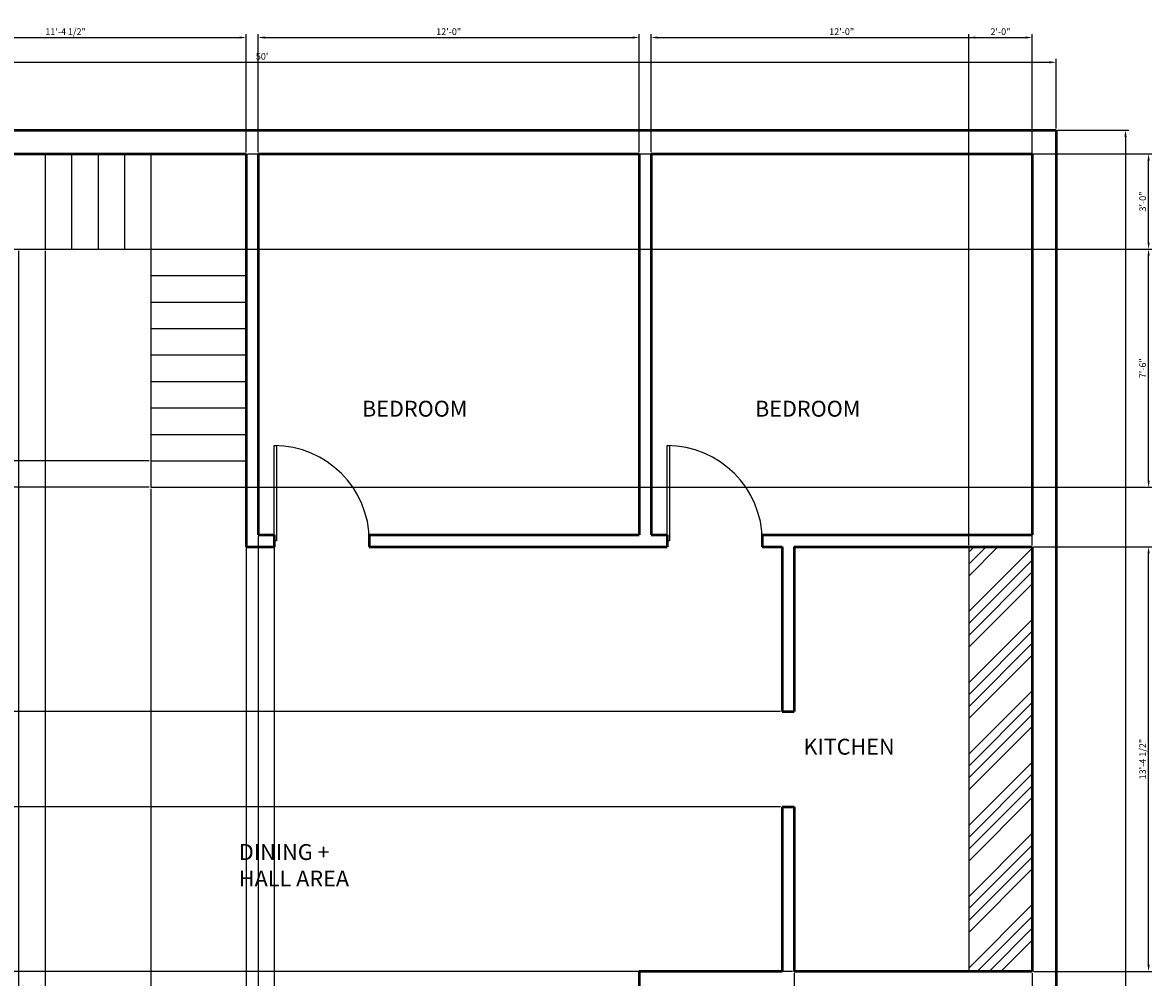
# Model space of a CAD drawing. Units: inches. Extents: x 877 to 2164, y 771 to 1603.
# Tile 4 of 6: x 1281 to 1709, y 1177 to 1538. Entities that reach past the tile are written whole.
import ezdxf

# ---------------------------------------------------------------- set-up
doc = ezdxf.new("R2010")
doc.units = ezdxf.units.IN
for name, color, linetype, lineweight in [('A-ANNO-DIMS', 2, 'Continuous', 18), ('A-AREA-IDEN', 7, 'Continuous', 25), ('A-DOOR', 5, 'Continuous', 25), ('A-FLOR-CASE', 8, 'Continuous', 25), ('A-FLOR-CASE-PATT', 252, 'Continuous', 13), ('A-FLOR-STRS', 7, 'Continuous', 25), ('A-WALL', 7, 'Continuous', 50)]:
    doc.layers.add(name, color=color, linetype=linetype, lineweight=lineweight)
doc.styles.get("Standard").update_dxf_attribs({"font": 'arial.ttf'})
doc.dimstyles.new('ISO-25', dxfattribs={"dimtxt": 2.5, "dimasz": 2.5, "dimexe": 1.25, "dimexo": 0.625, "dimtad": 1, "dimdec": 0, "dimlunit": 4, "dimtxsty": 'Standard', "dimcen": 2.5, "dimadec": 0, "dimazin": 0, "dimtfac": 1, "dimtdec": 0, "dimtmove": 0, "dimatfit": 3, "dimfxl": 1, "dimarcsym": 0})

# ---------------------------------------------------------------- blocks, each defined once
blk = doc.blocks.new('*D1')
at = {"layer": 'A-ANNO-DIMS', "color": 0, "lineweight": -2, "transparency": 16777216}
for p, q in [((1071.89, 1498.25), (1071.89, 1524.5)), ((1074.39, 1523.25), (1669.39, 1523.25)), ((1671.89, 1498.25), (1671.89, 1524.5))]:
    blk.add_line(p, q, dxfattribs=at)
at = {"layer": 'A-ANNO-DIMS', "color": 0, "transparency": 16777216}
for points in [[(1074.39, 1523.66), (1074.39, 1522.83), (1071.89, 1523.25)], [(1669.39, 1523.66), (1669.39, 1522.83), (1671.89, 1523.25)]]:
    blk.add_solid(points, dxfattribs=at)
at = {"layer": 'Defpoints', "color": 0, "transparency": 16777216}
for p in [(1671.89, 1523.25), (1071.89, 1497.62), (1671.89, 1497.62)]:
    blk.add_point(p, dxfattribs=at)
at = {"layer": 'A-ANNO-DIMS', "color": 0, "transparency": 16777216, "insert": (1371.89, 1525.15), "char_height": 2.5, "attachment_point": 5}
blk.add_mtext("50'", dxfattribs=at)
blk = doc.blocks.new('*D2')
at = {"layer": 'A-ANNO-DIMS', "color": 0, "lineweight": -2, "transparency": 16777216}
for p, q in [((1672.52, 1497.62), (1699.4, 1497.62)), ((1698.15, 1495.12), (1698.15, 840.12)), ((1672.52, 837.62), (1699.4, 837.62))]:
    blk.add_line(p, q, dxfattribs=at)
at = {"layer": 'A-ANNO-DIMS', "color": 0, "transparency": 16777216}
for points in [[(1697.73, 1495.12), (1698.57, 1495.12), (1698.15, 1497.62)], [(1697.73, 840.12), (1698.57, 840.12), (1698.15, 837.62)]]:
    blk.add_solid(points, dxfattribs=at)
at = {"layer": 'Defpoints', "color": 0, "transparency": 16777216}
for p in [(1671.89, 1497.62), (1671.89, 837.62), (1698.15, 837.62)]:
    blk.add_point(p, dxfattribs=at)
at = {"layer": 'A-ANNO-DIMS', "color": 0, "transparency": 16777216, "insert": (1696.26, 1167.62), "char_height": 2.5, "attachment_point": 5, "rotation": 90}
blk.add_mtext("55'", dxfattribs=at)
blk = doc.blocks.new('DOOR-SINGLE-36IN')
blk.add_lwpolyline([(0, 0), (0, 1), (36, 1), (36, 0)], close=True)
blk.add_arc((36, 0), 36, 90, 180)
blk = doc.blocks.new('*D11')
at = {"layer": 'A-ANNO-DIMS', "color": 0, "lineweight": -2, "transparency": 16777216}
for p, q in [((1229.39, 1489.25), (1229.39, 1533.85)), ((1231.89, 1532.6), (1363.39, 1532.6)), ((1365.89, 1489.25), (1365.89, 1533.85))]:
    blk.add_line(p, q, dxfattribs=at)
at = {"layer": 'A-ANNO-DIMS', "color": 0, "transparency": 16777216}
for points in [[(1231.89, 1533.01), (1231.89, 1532.18), (1229.39, 1532.6)], [(1363.39, 1533.01), (1363.39, 1532.18), (1365.89, 1532.6)]]:
    blk.add_solid(points, dxfattribs=at)
at = {"layer": 'Defpoints', "color": 0, "transparency": 16777216}
for p in [(1365.89, 1532.6), (1229.39, 1488.62), (1365.89, 1488.62)]:
    blk.add_point(p, dxfattribs=at)
at = {"layer": 'A-ANNO-DIMS', "color": 0, "transparency": 16777216, "insert": (1297.64, 1534.51), "char_height": 2.5, "attachment_point": 5}
blk.add_mtext('11\'-4 1/2"', dxfattribs=at)
blk = doc.blocks.new('*D12')
at = {"layer": 'A-ANNO-DIMS', "color": 0, "lineweight": -2, "transparency": 16777216}
for p, q in [((1370.39, 1489.25), (1370.39, 1533.85)), ((1372.89, 1532.6), (1511.89, 1532.6)), ((1514.39, 1489.25), (1514.39, 1533.85))]:
    blk.add_line(p, q, dxfattribs=at)
at = {"layer": 'A-ANNO-DIMS', "color": 0, "transparency": 16777216}
for points in [[(1372.89, 1533.01), (1372.89, 1532.18), (1370.39, 1532.6)], [(1511.89, 1533.01), (1511.89, 1532.18), (1514.39, 1532.6)]]:
    blk.add_solid(points, dxfattribs=at)
at = {"layer": 'Defpoints', "color": 0, "transparency": 16777216}
for p in [(1514.39, 1532.6), (1370.39, 1488.62), (1514.39, 1488.62)]:
    blk.add_point(p, dxfattribs=at)
at = {"layer": 'A-ANNO-DIMS', "color": 0, "transparency": 16777216, "insert": (1442.39, 1534.5), "char_height": 2.5, "attachment_point": 5}
blk.add_mtext('12\'-0"', dxfattribs=at)
blk = doc.blocks.new('*D13')
at = {"layer": 'A-ANNO-DIMS', "color": 0, "lineweight": -2, "transparency": 16777216}
for p, q in [((1518.89, 1489.25), (1518.89, 1533.85)), ((1521.39, 1532.6), (1660.39, 1532.6)), ((1662.89, 1489.25), (1662.89, 1533.85))]:
    blk.add_line(p, q, dxfattribs=at)
at = {"layer": 'A-ANNO-DIMS', "color": 0, "transparency": 16777216}
for points in [[(1521.39, 1533.01), (1521.39, 1532.18), (1518.89, 1532.6)], [(1660.39, 1533.01), (1660.39, 1532.18), (1662.89, 1532.6)]]:
    blk.add_solid(points, dxfattribs=at)
at = {"layer": 'Defpoints', "color": 0, "transparency": 16777216}
for p in [(1662.89, 1532.6), (1518.89, 1488.62), (1662.89, 1488.62)]:
    blk.add_point(p, dxfattribs=at)
at = {"layer": 'A-ANNO-DIMS', "color": 0, "transparency": 16777216, "insert": (1590.89, 1534.5), "char_height": 2.5, "attachment_point": 5}
blk.add_mtext('12\'-0"', dxfattribs=at)
blk = doc.blocks.new('*D17')
at = {"layer": 'A-ANNO-DIMS', "color": 0, "lineweight": -2, "transparency": 16777216}
for p, q in [((1638.89, 1340.75), (1638.89, 1533.85)), ((1641.39, 1532.6), (1660.39, 1532.6)), ((1662.89, 1340.75), (1662.89, 1533.85))]:
    blk.add_line(p, q, dxfattribs=at)
at = {"layer": 'A-ANNO-DIMS', "color": 0, "transparency": 16777216}
for points in [[(1641.39, 1533.01), (1641.39, 1532.18), (1638.89, 1532.6)], [(1660.39, 1533.01), (1660.39, 1532.18), (1662.89, 1532.6)]]:
    blk.add_solid(points, dxfattribs=at)
at = {"layer": 'Defpoints', "color": 0, "transparency": 16777216}
for p in [(1662.89, 1532.6), (1638.89, 1340.12), (1662.89, 1340.12)]:
    blk.add_point(p, dxfattribs=at)
at = {"layer": 'A-ANNO-DIMS', "color": 0, "transparency": 16777216, "insert": (1650.89, 1534.5), "char_height": 2.5, "attachment_point": 5}
blk.add_mtext('2\'-0"', dxfattribs=at)
blk = doc.blocks.new('*D18')
at = {"layer": 'A-ANNO-DIMS', "color": 0, "lineweight": -2, "transparency": 16777216}
for p, q in [((1572.89, 1179), (1572.89, 771.4)), ((1662.89, 1179), (1662.89, 771.4)), ((1575.39, 772.65), (1660.39, 772.65))]:
    blk.add_line(p, q, dxfattribs=at)
at = {"layer": 'A-ANNO-DIMS', "color": 0, "transparency": 16777216}
for points in [[(1575.39, 773.06), (1575.39, 772.23), (1572.89, 772.65)], [(1660.39, 773.06), (1660.39, 772.23), (1662.89, 772.65)]]:
    blk.add_solid(points, dxfattribs=at)
at = {"layer": 'Defpoints', "color": 0, "transparency": 16777216}
for p in [(1572.89, 1179.62), (1662.89, 1179.62), (1662.89, 772.65)]:
    blk.add_point(p, dxfattribs=at)
at = {"layer": 'A-ANNO-DIMS', "color": 0, "transparency": 16777216, "insert": (1617.89, 774.55), "char_height": 2.5, "attachment_point": 5}
blk.add_mtext('7\'-6"', dxfattribs=at)
blk = doc.blocks.new('*D19')
at = {"layer": 'A-ANNO-DIMS', "color": 0, "lineweight": -2, "transparency": 16777216}
for p, q in [((1567.77, 1277.87), (1035.67, 1277.87)), ((1036.92, 1244.37), (1036.92, 1275.37)), ((1567.77, 1241.87), (1035.67, 1241.87))]:
    blk.add_line(p, q, dxfattribs=at)
at = {"layer": 'A-ANNO-DIMS', "color": 0, "transparency": 16777216}
for points in [[(1036.5, 1275.37), (1037.34, 1275.37), (1036.92, 1277.87)], [(1036.5, 1244.37), (1037.34, 1244.37), (1036.92, 1241.87)]]:
    blk.add_solid(points, dxfattribs=at)
at = {"layer": 'Defpoints', "color": 0, "transparency": 16777216}
for p in [(1036.92, 1277.87), (1568.39, 1277.87), (1568.39, 1241.87)]:
    blk.add_point(p, dxfattribs=at)
at = {"layer": 'A-ANNO-DIMS', "color": 0, "transparency": 16777216, "insert": (1035.02, 1259.87), "char_height": 2.5, "attachment_point": 5, "rotation": 90}
blk.add_mtext('3\'-0"', dxfattribs=at)
blk = doc.blocks.new('*D20')
at = {"layer": 'A-ANNO-DIMS', "color": 0, "lineweight": -2, "transparency": 16777216}
for p, q in [((1567.77, 1241.87), (1035.67, 1241.87)), ((1036.92, 1182.12), (1036.92, 1239.37)), ((1572.27, 1179.62), (1035.67, 1179.62))]:
    blk.add_line(p, q, dxfattribs=at)
at = {"layer": 'A-ANNO-DIMS', "color": 0, "transparency": 16777216}
for points in [[(1036.5, 1239.37), (1037.34, 1239.37), (1036.92, 1241.87)], [(1036.5, 1182.12), (1037.34, 1182.12), (1036.92, 1179.62)]]:
    blk.add_solid(points, dxfattribs=at)
at = {"layer": 'Defpoints', "color": 0, "transparency": 16777216}
for p in [(1036.92, 1241.87), (1568.39, 1241.87), (1572.89, 1179.62)]:
    blk.add_point(p, dxfattribs=at)
at = {"layer": 'A-ANNO-DIMS', "color": 0, "transparency": 16777216, "insert": (1035, 1210.75), "char_height": 2.5, "attachment_point": 5, "rotation": 90}
blk.add_mtext('5\'-2 1/2"', dxfattribs=at)
blk = doc.blocks.new('*D21')
at = {"layer": 'A-ANNO-DIMS', "color": 0, "lineweight": -2, "transparency": 16777216}
for p, q in [((1663.52, 1340.12), (1708.12, 1340.12)), ((1706.87, 1182.12), (1706.87, 1337.62)), ((1663.52, 1179.62), (1708.12, 1179.62))]:
    blk.add_line(p, q, dxfattribs=at)
at = {"layer": 'A-ANNO-DIMS', "color": 0, "transparency": 16777216}
for points in [[(1706.45, 1337.62), (1707.29, 1337.62), (1706.87, 1340.12)], [(1706.45, 1182.12), (1707.29, 1182.12), (1706.87, 1179.62)]]:
    blk.add_solid(points, dxfattribs=at)
at = {"layer": 'Defpoints', "color": 0, "transparency": 16777216}
for p in [(1662.89, 1340.12), (1706.87, 1340.12), (1662.89, 1179.62)]:
    blk.add_point(p, dxfattribs=at)
at = {"layer": 'A-ANNO-DIMS', "color": 0, "transparency": 16777216, "insert": (1704.95, 1259.87), "char_height": 2.5, "attachment_point": 5, "rotation": 90}
blk.add_mtext('13\'-4 1/2"', dxfattribs=at)
blk = doc.blocks.new('*D38')
at = {"layer": 'A-ANNO-DIMS', "color": 0, "lineweight": -2, "transparency": 16777216}
for p, q in [((1366.52, 1452.62), (1708.12, 1452.62)), ((1706.87, 1365.12), (1706.87, 1450.12)), ((1366.52, 1362.62), (1708.12, 1362.62))]:
    blk.add_line(p, q, dxfattribs=at)
at = {"layer": 'A-ANNO-DIMS', "color": 0, "transparency": 16777216}
for points in [[(1706.45, 1450.12), (1707.29, 1450.12), (1706.87, 1452.62)], [(1706.45, 1365.12), (1707.29, 1365.12), (1706.87, 1362.62)]]:
    blk.add_solid(points, dxfattribs=at)
at = {"layer": 'Defpoints', "color": 0, "transparency": 16777216}
for p in [(1365.89, 1452.62), (1706.87, 1452.62), (1365.89, 1362.62)]:
    blk.add_point(p, dxfattribs=at)
at = {"layer": 'A-ANNO-DIMS', "color": 0, "transparency": 16777216, "insert": (1704.97, 1407.62), "char_height": 2.5, "attachment_point": 5, "rotation": 90}
blk.add_mtext('7\'-6"', dxfattribs=at)
blk = doc.blocks.new('*D39')
at = {"layer": 'A-ANNO-DIMS', "color": 0, "lineweight": -2, "transparency": 16777216}
for p, q in [((1366.52, 1488.62), (1708.12, 1488.62)), ((1706.87, 1455.12), (1706.87, 1486.12)), ((1366.52, 1452.62), (1708.12, 1452.62))]:
    blk.add_line(p, q, dxfattribs=at)
at = {"layer": 'A-ANNO-DIMS', "color": 0, "transparency": 16777216}
for points in [[(1706.45, 1486.12), (1707.29, 1486.12), (1706.87, 1488.62)], [(1706.45, 1455.12), (1707.29, 1455.12), (1706.87, 1452.62)]]:
    blk.add_solid(points, dxfattribs=at)
at = {"layer": 'Defpoints', "color": 0, "transparency": 16777216}
for p in [(1365.89, 1488.62), (1706.87, 1488.62), (1365.89, 1452.62)]:
    blk.add_point(p, dxfattribs=at)
at = {"layer": 'A-ANNO-DIMS', "color": 0, "transparency": 16777216, "insert": (1704.97, 1470.62), "char_height": 2.5, "attachment_point": 5, "rotation": 90}
blk.add_mtext('3\'-0"', dxfattribs=at)
blk = doc.blocks.new('*D41')
at = {"layer": 'A-ANNO-DIMS', "color": 0, "lineweight": -2, "transparency": 16777216}
for p, q in [((1329.27, 1372.62), (1035.67, 1372.62)), ((1036.92, 1365.12), (1036.92, 1370.12)), ((1329.27, 1362.62), (1035.67, 1362.62))]:
    blk.add_line(p, q, dxfattribs=at)
at = {"layer": 'A-ANNO-DIMS', "color": 0, "transparency": 16777216}
for points in [[(1036.5, 1370.12), (1037.34, 1370.12), (1036.92, 1372.62)], [(1036.5, 1365.12), (1037.34, 1365.12), (1036.92, 1362.62)]]:
    blk.add_solid(points, dxfattribs=at)
at = {"layer": 'Defpoints', "color": 0, "transparency": 16777216}
for p in [(1036.92, 1372.62), (1329.89, 1372.62), (1329.89, 1362.62)]:
    blk.add_point(p, dxfattribs=at)
at = {"layer": 'A-ANNO-DIMS', "color": 0, "transparency": 16777216, "insert": (1035.02, 1367.62), "char_height": 2.5, "attachment_point": 5, "rotation": 90}
blk.add_mtext('0\'-10"', dxfattribs=at)
blk = doc.blocks.new('*D42')
at = {"layer": 'A-ANNO-DIMS', "color": 0, "lineweight": -2, "transparency": 16777216}
for p, q in [((1329.89, 1362), (1329.89, 771.4)), ((1365.89, 1362), (1365.89, 771.4)), ((1332.39, 772.65), (1363.39, 772.65))]:
    blk.add_line(p, q, dxfattribs=at)
at = {"layer": 'A-ANNO-DIMS', "color": 0, "transparency": 16777216}
for points in [[(1332.39, 773.06), (1332.39, 772.23), (1329.89, 772.65)], [(1363.39, 773.06), (1363.39, 772.23), (1365.89, 772.65)]]:
    blk.add_solid(points, dxfattribs=at)
at = {"layer": 'Defpoints', "color": 0, "transparency": 16777216}
for p in [(1329.89, 1362.62), (1365.89, 1362.62), (1365.89, 772.65)]:
    blk.add_point(p, dxfattribs=at)
at = {"layer": 'A-ANNO-DIMS', "color": 0, "transparency": 16777216, "insert": (1347.89, 774.55), "char_height": 2.5, "attachment_point": 5}
blk.add_mtext('3\'-0"', dxfattribs=at)
blk = doc.blocks.new('*D44')
at = {"layer": 'A-ANNO-DIMS', "color": 0, "lineweight": -2, "transparency": 16777216}
for p, q in [((1279.89, 1452), (1279.89, 771.4)), ((1289.89, 1452), (1289.89, 771.4)), ((1282.39, 772.65), (1287.39, 772.65))]:
    blk.add_line(p, q, dxfattribs=at)
at = {"layer": 'A-ANNO-DIMS', "color": 0, "transparency": 16777216}
for points in [[(1282.39, 773.06), (1282.39, 772.23), (1279.89, 772.65)], [(1287.39, 773.06), (1287.39, 772.23), (1289.89, 772.65)]]:
    blk.add_solid(points, dxfattribs=at)
at = {"layer": 'Defpoints', "color": 0, "transparency": 16777216}
for p in [(1279.89, 1452.62), (1289.89, 1452.62), (1289.89, 772.65)]:
    blk.add_point(p, dxfattribs=at)
at = {"layer": 'A-ANNO-DIMS', "color": 0, "transparency": 16777216, "insert": (1284.89, 774.55), "char_height": 2.5, "attachment_point": 5}
blk.add_mtext('0\'-10"', dxfattribs=at)
blk = doc.blocks.new('*D46')
at = {"layer": 'A-ANNO-DIMS', "color": 0, "lineweight": -2, "transparency": 16777216}
for p, q in [((1370.39, 1344), (1370.39, 771.4)), ((1376.39, 1344), (1376.39, 771.4)), ((1367.89, 772.65), (1365.39, 772.65)), ((1370.39, 772.65), (1376.39, 772.65)), ((1378.89, 772.65), (1389.29, 772.65))]:
    blk.add_line(p, q, dxfattribs=at)
at = {"layer": 'A-ANNO-DIMS', "color": 0, "transparency": 16777216}
for points in [[(1367.89, 773.06), (1367.89, 772.23), (1370.39, 772.65)], [(1378.89, 773.06), (1378.89, 772.23), (1376.39, 772.65)]]:
    blk.add_solid(points, dxfattribs=at)
at = {"layer": 'Defpoints', "color": 0, "transparency": 16777216}
for p in [(1370.39, 1344.62), (1376.39, 1344.62), (1376.39, 772.65)]:
    blk.add_point(p, dxfattribs=at)
at = {"layer": 'A-ANNO-DIMS', "color": 0, "transparency": 16777216, "insert": (1385.34, 774.55), "char_height": 2.5, "attachment_point": 5}
blk.add_mtext('0\'-6"', dxfattribs=at)

msp = doc.modelspace()

# ---------------------------------------------------------------- hatches: boundary and pattern name
at = {"layer": 'A-FLOR-CASE-PATT'}
h = msp.add_hatch(dxfattribs=at)
h.set_pattern_fill('ANSI34', color=256)
h.paths.add_polyline_path([(1662.89, 1340.12), (1638.89, 1340.12), (1638.89, 1179.62), (1662.89, 1179.62)])

# ---------------------------------------------------------------- linework, layer by layer
at = {"layer": 'A-FLOR-CASE'}
msp.add_line((1638.89, 1340.12), (1638.89, 1179.62), dxfattribs=at)
at = {"layer": 'A-FLOR-STRS'}
for p, q in [((1289.89, 1488.62), (1289.89, 1452.62)), ((1299.89, 1488.62), (1299.89, 1452.62)), ((1309.89, 1488.62), (1309.89, 1452.62)), ((1319.89, 1488.62), (1319.89, 1452.62)), ((1329.89, 1488.62), (1329.89, 1362.62)), ((1229.39, 1452.62), (1365.89, 1452.62)), ((1329.89, 1442.62), (1365.89, 1442.62)), ((1329.89, 1432.62), (1365.89, 1432.62)), ((1329.89, 1422.62), (1365.89, 1422.62)), ((1329.89, 1412.62), (1365.89, 1412.62)), ((1329.89, 1402.62), (1365.89, 1402.62)), ((1329.89, 1392.62), (1365.89, 1392.62)), ((1329.89, 1382.62), (1365.89, 1382.62)), ((1329.89, 1372.62), (1365.89, 1372.62)), ((1329.89, 1362.62), (1365.89, 1362.62))]:
    msp.add_line(p, q, dxfattribs=at)
at = {"layer": 'A-WALL'}
for p, q in [((1071.89, 1497.62), (1671.89, 1497.62)), ((1671.89, 1497.62), (1671.89, 837.62)), ((1229.39, 1488.62), (1365.89, 1488.62)), ((1365.89, 1488.62), (1365.89, 1340.12)), ((1370.39, 1488.62), (1370.39, 1344.62)), ((1370.39, 1488.62), (1514.39, 1488.62)), ((1514.39, 1488.62), (1514.39, 1344.62)), ((1518.89, 1488.62), (1518.89, 1344.62)), ((1518.89, 1488.62), (1662.89, 1488.62)), ((1662.89, 1488.62), (1662.89, 1344.62)), ((1370.39, 1344.62), (1376.39, 1344.62)), ((1376.39, 1344.62), (1376.39, 1340.12)), ((1412.39, 1344.62), (1412.39, 1340.12)), ((1412.39, 1344.62), (1514.39, 1344.62)), ((1518.89, 1344.62), (1524.89, 1344.62)), ((1524.89, 1344.62), (1524.89, 1340.12)), ((1560.89, 1344.62), (1560.89, 1340.12)), ((1560.89, 1344.62), (1662.89, 1344.62)), ((1365.89, 1340.12), (1376.39, 1340.12)), ((1412.39, 1340.12), (1524.89, 1340.12)), ((1560.89, 1340.12), (1568.39, 1340.12)), ((1568.39, 1340.12), (1568.39, 1277.87)), ((1572.89, 1340.12), (1572.89, 1277.87)), ((1572.89, 1340.12), (1662.89, 1340.12)), ((1662.89, 1340.12), (1662.89, 1179.62)), ((1568.39, 1277.87), (1572.89, 1277.87)), ((1568.39, 1241.87), (1568.39, 1179.62)), ((1568.39, 1241.87), (1572.89, 1241.87)), ((1572.89, 1241.87), (1572.89, 1179.62)), ((1514.39, 1179.62), (1514.39, 1169.12)), ((1568.39, 1179.62), (1514.39, 1179.62)), ((1662.89, 1179.62), (1572.89, 1179.62))]:
    msp.add_line(p, q, dxfattribs=at)

# ---------------------------------------------------------------- block references
at = {"layer": 'A-DOOR', "rotation": 269.9999999999998}
for p in [(1376.39, 1378.37), (1524.89, 1378.37)]:
    msp.add_blockref('DOOR-SINGLE-36IN', p, dxfattribs=at)

# ---------------------------------------------------------------- texts
at = {"layer": 'A-AREA-IDEN', "char_height": 6, "attachment_point": 1}
for s, insert in [('BEDROOM', (1409.64, 1395.31)), ('BEDROOM', (1558.14, 1395.31)), ('KITCHEN', (1576.41, 1267.56)), ('DINING + HALL AREA', (1363.11, 1227.75))]:
    msp.add_mtext_dynamic_manual_height_columns(s, width=54.8109, gutter_width=12.5, heights=[0], dxfattribs=dict(at, insert=insert))

# ---------------------------------------------------------------- dimensions: what is measured, and where the dimension line sits
at = {"layer": 'A-ANNO-DIMS'}
for base, p1, p2, override, picture, middle in [((1365.89, 1532.6), (1229.39, 1488.62), (1365.89, 1488.62), {"dimdec": 1, "dimlfac": 1, "dimrnd": 0, "dimzin": 1, "dimdsep": 46, "dimlunit": 4, "dimfrac": 2}, '*D11', (1297.64, 1534.51)), ((1514.39, 1532.6), (1370.39, 1488.62), (1514.39, 1488.62), {"dimdec": 1, "dimlfac": 1, "dimrnd": 0, "dimzin": 1, "dimdsep": 46, "dimlunit": 4, "dimfrac": 2}, '*D12', (1442.39, 1534.5)), ((1662.89, 1532.6), (1518.89, 1488.62), (1662.89, 1488.62), {"dimdec": 1, "dimlfac": 1, "dimrnd": 0, "dimzin": 1, "dimdsep": 46, "dimlunit": 4, "dimfrac": 2}, '*D13', (1590.89, 1534.5)), ((1662.89, 1532.6), (1638.89, 1340.12), (1662.89, 1340.12), {"dimdec": 1, "dimlfac": 1, "dimrnd": 0, "dimzin": 1, "dimdsep": 46, "dimlunit": 4, "dimfrac": 2}, '*D17', (1650.89, 1534.5)), ((1671.89, 1523.25), (1071.89, 1497.62), (1671.89, 1497.62), {"dimclrd": 0, "dimclre": 0, "dimclrt": 0}, '*D1', (1371.89, 1525.15)), ((1289.89, 772.65), (1279.89, 1452.62), (1289.89, 1452.62), {"dimdec": 1, "dimlfac": 1, "dimrnd": 0, "dimzin": 1, "dimdsep": 46, "dimlunit": 4, "dimfrac": 2}, '*D44', (1284.89, 774.55)), ((1365.89, 772.65), (1329.89, 1362.62), (1365.89, 1362.62), {"dimdec": 1, "dimlfac": 1, "dimrnd": 0, "dimzin": 1, "dimdsep": 46, "dimlunit": 4, "dimfrac": 2}, '*D42', (1347.89, 774.55)), ((1376.39, 772.65), (1370.39, 1344.62), (1376.39, 1344.62), {"dimdec": 1, "dimlfac": 1, "dimrnd": 0, "dimzin": 1, "dimdsep": 46, "dimlunit": 4, "dimfrac": 2}, '*D46', (1385.34, 774.55)), ((1662.89, 772.65), (1572.89, 1179.62), (1662.89, 1179.62), {"dimdec": 1, "dimlfac": 1, "dimrnd": 0, "dimzin": 1, "dimdsep": 46, "dimlunit": 4, "dimfrac": 2}, '*D18', (1617.89, 774.55))]:
    dim = msp.add_linear_dim(base=base, p1=p1, p2=p2, dimstyle='ISO-25', override=override, dxfattribs=at)
    dim.commit()
    dim.dimension.update_dxf_attribs({"geometry": picture, "text_midpoint": middle})
for base, p1, p2, override, picture, middle in [((1698.15, 837.62), (1671.89, 1497.62), (1671.89, 837.62), {"dimclrd": 0, "dimclre": 0, "dimclrt": 0}, '*D2', (1696.26, 1167.62)), ((1706.87, 1488.62), (1365.89, 1452.62), (1365.89, 1488.62), {"dimdec": 1, "dimlfac": 1, "dimrnd": 0, "dimzin": 1, "dimdsep": 46, "dimlunit": 4, "dimfrac": 2}, '*D39', (1704.97, 1470.62)), ((1706.87, 1452.62), (1365.89, 1362.62), (1365.89, 1452.62), {"dimdec": 1, "dimlfac": 1, "dimrnd": 0, "dimzin": 1, "dimdsep": 46, "dimlunit": 4, "dimfrac": 2}, '*D38', (1704.97, 1407.62)), ((1036.92, 1372.62), (1329.89, 1362.62), (1329.89, 1372.62), {"dimdec": 1, "dimlfac": 1, "dimrnd": 0, "dimzin": 1, "dimdsep": 46, "dimlunit": 4, "dimfrac": 2}, '*D41', (1035.02, 1367.62)), ((1706.87, 1340.12), (1662.89, 1179.62), (1662.89, 1340.12), {"dimdec": 1, "dimlfac": 1, "dimrnd": 0, "dimzin": 1, "dimdsep": 46, "dimlunit": 4, "dimfrac": 2}, '*D21', (1704.95, 1259.87)), ((1036.92, 1277.87), (1568.39, 1241.87), (1568.39, 1277.87), {"dimdec": 1, "dimlfac": 1, "dimrnd": 0, "dimzin": 1, "dimdsep": 46, "dimlunit": 4, "dimfrac": 2}, '*D19', (1035.02, 1259.87)), ((1036.91999, 1241.870352), (1572.89499, 1179.620352), (1568.39499, 1241.870352), {"dimdec": 1, "dimlfac": 1, "dimrnd": 0, "dimzin": 1, "dimdsep": 46, "dimlunit": 4, "dimfrac": 2}, '*D20', (1035.00235698, 1210.745352))]:
    dim = msp.add_linear_dim(base=base, p1=p1, p2=p2, angle=90, dimstyle='ISO-25', override=override, dxfattribs=at)
    dim.commit()
    dim.dimension.update_dxf_attribs({"geometry": picture, "text_midpoint": middle})

doc.saveas('drawing.dxf')
